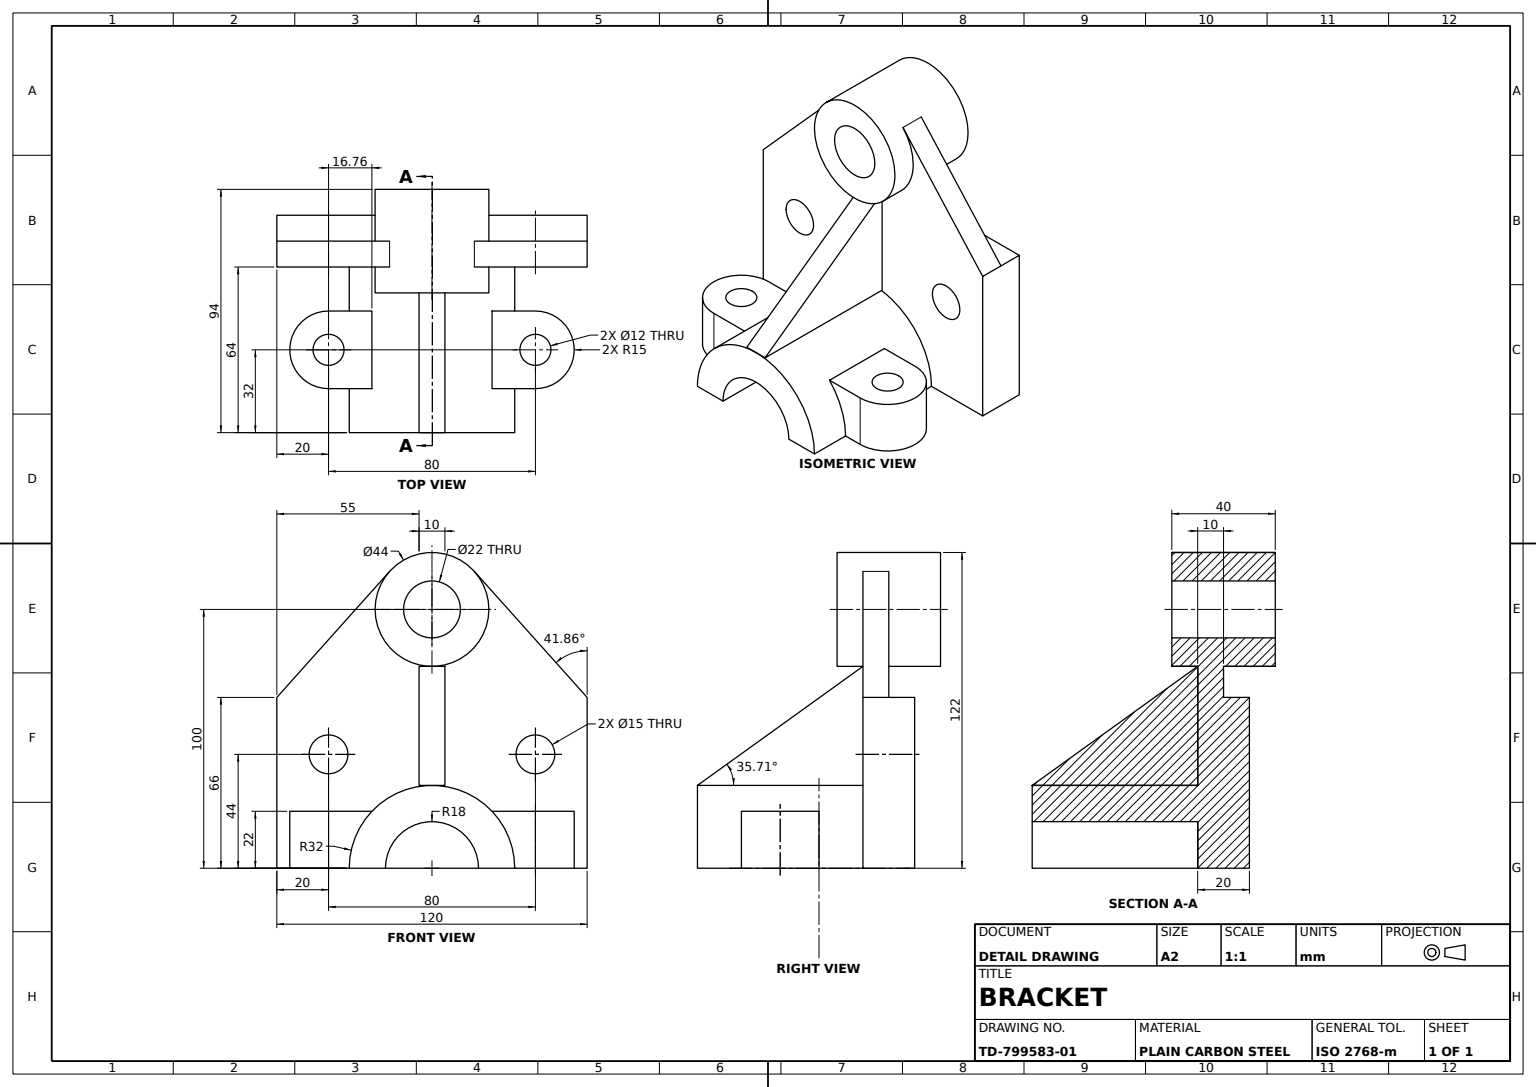
SolidWorks part; units mm, degrees
material "Plain Carbon Steel"
ref_plane "Front Plane" through (0, 0, 0) normal (0, 0, 1) x (1, 0, 0)
ref_plane "Top Plane" through (0, 0, 0) normal (0, 1, 0) x (1, 0, 0)
ref_plane "Right Plane" through (0, 0, 0) normal (1, 0, 0) x (0, 0, -1)
sketch "Base Plate Sketch" plane through (0, 0, 0) normal (0, 0, 1) x (1, 0, 0)
  line L0 (0, 0) -> (120, 0)
  line L1 (120, 0) -> (120, 66)
  line L2 (120, 66) -> (0, 66)
  line L3 (0, 66) -> (0, 0)
  dimension "D1" = 120
  dimension "D2" = 66
  dimension "D3" = 120
extrude "Base Plate" add sketch "Base Plate Sketch" against normal blind 20
sketch "Saddle Boss Sketch" plane through (0, 0, 0) normal (0, 0, 1) x (1, 0, 0)
  line L0 (0, 0) -> (120, 0) construction
  line L1 (28, 0) -> (92, 0)
  arc A0 (92, 0) -> (28, 0) centre (60, 0) ccw
  dimension "D1" = 32
extrude "Saddle Boss R32" add sketch "Saddle Boss Sketch" along normal blind 64
sketch "Saddle Bore Sketch" plane through (0, 0, 64) normal (0, 0, 1) x (1, 0, 0)
  line L0 (28, 0) -> (92, 0) construction
  line L1 (42, 0) -> (78, 0)
  arc A0 (78, 0) -> (42, 0) centre (60, 0) ccw
  dimension "D1" = 18
extrude "Saddle Bore R18" cut sketch "Saddle Bore Sketch" against normal blind 64
sketch "Upright Plate Sketch" plane through (0, 0, 0) normal (0, 0, 1) x (1, 0, 0)
  line L0 (60, 0) -> (60, 100)
  line L1 (42, 0) -> (78, 0) construction
  line L2 (0, 66) -> (43.6144, 114.6804)
  line L3 (120, 66) -> (76.3856, 114.6804)
  line L4 (0, 66) -> (120, 66)
  circle A0 centre (60, 100) radius 22
  dimension "D2" = 44
  dimension "D1" = 100
extrude "Upright Plate" add sketch "Upright Plate Sketch" against normal blind 10
sketch "Eye Boss Front Sketch" plane through (0, 0, 0) normal (0, 0, 1) x (1, 0, 0)
  circle A0 centre (60, 100) radius 22
  dimension "D1" = 44
extrude "Eye Boss Front Ø44" add sketch "Eye Boss Front Sketch" along normal blind 10
sketch "Eye Boss Rear Sketch" plane through (0, 0, -10) normal (0, 0, -1) x (-1, 0, 0)
  circle A0 centre (-60, 100) radius 22
  dimension "D1" = 44
extrude "Eye Boss Rear Ø44" add sketch "Eye Boss Rear Sketch" along normal blind 20
sketch "Eye Bore Sketch" plane through (0, 0, 10) normal (0, 0, 1) x (1, 0, 0)
  circle A0 centre (60, 100) radius 11
  dimension "D1" = 22
extrude "Eye Bore Ø22" cut sketch "Eye Bore Sketch" against normal blind 50
sketch "Mounting Lugs Sketch" plane through (0, 0, 0) normal (0, -1, 0) x (1, 0, 0)
  line L0 (28, 0) -> (28, 32)
  line L1 (60, 32) -> (100, 32)
  line L2 (28, 64) -> (28, 0) construction
  line L3 (60, 0) -> (60, 64)
  line L4 (42, 0) -> (78, 0) construction
  line L5 (78, 64) -> (42, 64) construction
  line L6 (60, 32) -> (20, 32)
  line L13 (20, 47) -> (42, 47)
  line L14 (42, 0) -> (42, 64) construction
  line L15 (42, 47) -> (42, 17)
  line L16 (42, 17) -> (20, 17)
  line L17 (100, 47) -> (78, 47)
  line L18 (78, 0) -> (78, 64) construction
  line L19 (78, 47) -> (78, 17)
  line L20 (78, 17) -> (100, 17)
  arc A0 (20, 47) -> (20, 17) centre (20, 32) ccw
  arc A1 (100, 17) -> (100, 47) centre (100, 32) ccw
  dimension "D3" = 15
  dimension "D5" = 15
  dimension "D1" = 32
  dimension "D2" = 40
  dimension "D4" = 40
extrude "Saddle Mounting Lugs" add sketch "Mounting Lugs Sketch" against normal blind 22
sketch "Plate Relief Sketch" plane through (0, 0, 0) normal (0, 0, 1) x (1, 0, 0)
  line L0 (60, 78) -> (60, 32)
  line L1 (60, 55) -> (55, 55)
  line L2 (60, 55) -> (65, 55)
  circle A0 centre (20, 44) radius 7.5
  circle A1 centre (100, 44) radius 7.5
  arc A2 (43.6144, 114.6804) -> (76.3856, 114.6804) centre (60, 100) ccw construction
  arc A3 (92, 0) -> (28, 0) centre (60, 0) ccw construction
  dimension "D1" = 15
  dimension "D2" = 15
  dimension "D3" = 44
  dimension "D4" = 5
  dimension "D5" = 35
  dimension "D6" = 5
  dimension "D7" = 35
  dimension "D8" = 44
extrude "Plate Relief Cut" cut sketch "Plate Relief Sketch" against normal blind 30 contours A0 | A1
sketch "Rib Block Sketch" plane through (0, 0, 0) normal (-1, 0, 0) x (0, 0, 1)
  line L0 (0, 78) -> (64, 32)
  line L1 (64, 32) -> (0, 32)
  line L2 (0, 32) -> (0, 78)
extrude "Rib Block" add sketch "Rib Block Sketch" against normal blind 120 separate body
sketch "Rib Trim Side A Sketch" plane through (0, 0, 0) normal (-1, 0, 0) x (0, 0, 1)
  line L0 (0, 78) -> (64, 32)
  line L1 (64, 32) -> (0, 32)
  line L2 (0, 32) -> (0, 78)
extrude "Rib Trim Side A" cut sketch "Rib Trim Side A Sketch" against normal blind 55
sketch "Rib Trim Side B Sketch" plane through (120, 0, 0) normal (1, 0, 0) x (0, 0, -1)
  line L0 (0, 78) -> (-64, 32)
  line L1 (-64, 32) -> (0, 32)
  line L2 (0, 32) -> (0, 78)
extrude "Rib Trim Side B" cut sketch "Rib Trim Side B Sketch" against normal blind 55
sketch "Lug Holes Sketch" plane through (0, 22, 0) normal (0, 1, 0) x (1, 0, 0)
  circle A0 centre (20, -32) radius 6
  circle A1 centre (100, -32) radius 6
  dimension "D1" = 12
  dimension "D2" = 12
extrude "Lug Holes 2xØ12" cut sketch "Lug Holes Sketch" against normal blind 55
